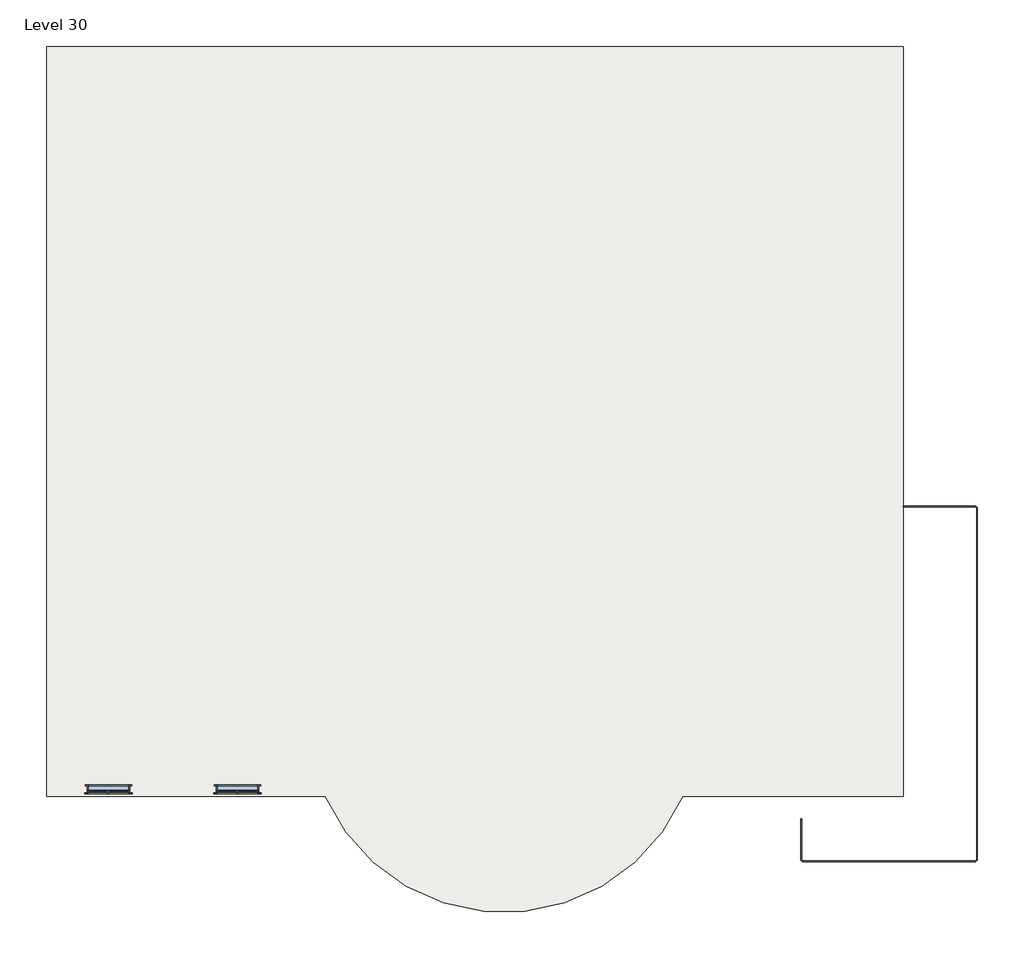
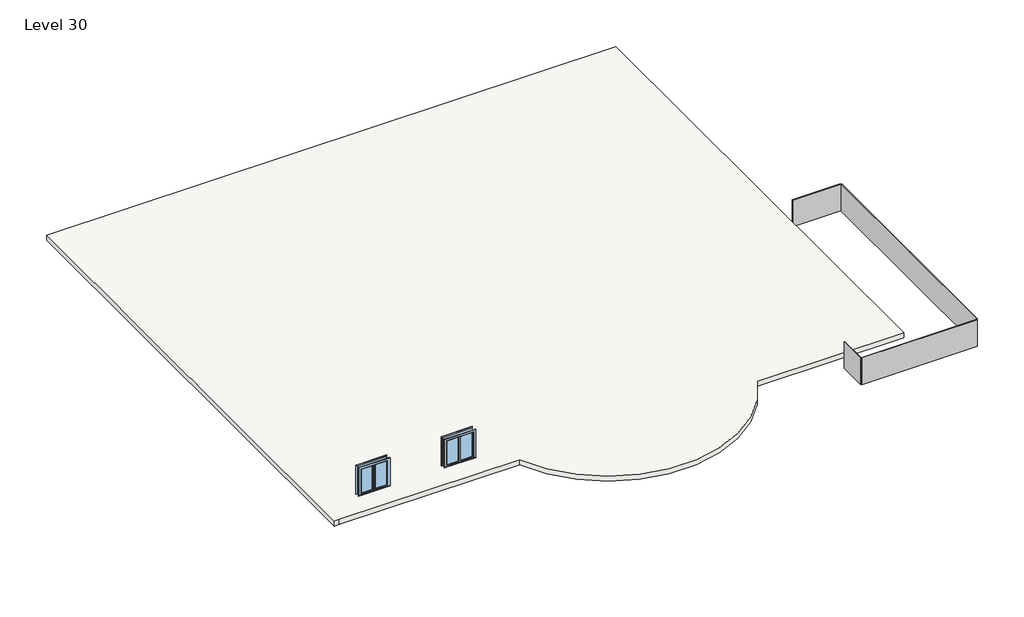
# One storey: 4 plates, 2 windows, 1 slab.
"""IFC4 building model written with IfcOpenShell, lengths in millimetres."""

from ifc_helpers import new_model, si_unit, point, frame, frame_2d, origin, place, context, project, spatial, polyline, circle_curve, trimmed, segment, composite_curve, outline, extrude, transform, mapped, element, save
from components import system_panel_glazed_4fcd3a06, system_panel_glazed_f6fb2dd6, system_panel_glazed_f39c722f, system_panel_glazed_542b97c0, window_0862ab64

model = new_model("IFC4")

# Units and contexts
model_context = context("Model", 3, world=origin())
ifc_project = project(units=[si_unit("LENGTHUNIT", "METRE", prefix="MILLI")], contexts=[model_context])

# Site, building, storey
site = spatial("IfcSite", under=ifc_project)
building = spatial("IfcBuilding", under=site)
storey = spatial("IfcBuildingStorey", under=building, Name="Level 30", Elevation=48920.4)

# Plates
placement = place(None, origin())
system_panel_glazed_shape = system_panel_glazed_4fcd3a06(model_context)
element("IfcPlate", 1, ObjectType="System Panel : Glazed", at=placement, inside=storey, context=model_context, shape_type="MappedRepresentation", body=[
    mapped(system_panel_glazed_shape, transform((9025.4464352, -5885.6278294, 48920.4), x_axis=(1.0, 0.0, 0.0), y_axis=(0.0, 1.0, 0.0), z_axis=(0.0, 0.0, 1.0))),
])
system_panel_glazed_2_shape = system_panel_glazed_f6fb2dd6(model_context)
element("IfcPlate", 2, ObjectType="System Panel : Glazed", at=placement, inside=storey, context=model_context, shape_type="MappedRepresentation", body=[
    mapped(system_panel_glazed_2_shape, transform((5082.0964352, -15423.3278294, 48920.4), x_axis=(0.0, 1.0, 0.0), y_axis=(-1.0, 0.0, 0.0), z_axis=(0.0, 0.0, 1.0))),
])
system_panel_glazed_3_shape = system_panel_glazed_f39c722f(model_context)
element("IfcPlate", 3, ObjectType="System Panel : Glazed", at=placement, inside=storey, context=model_context, shape_type="MappedRepresentation", body=[
    mapped(system_panel_glazed_3_shape, transform((10066.8464352, -10952.9278294, 48920.4), x_axis=(0.0, -1.0, 0.0), y_axis=(1.0, 0.0, 0.0), z_axis=(0.0, 0.0, 1.0))),
])
system_panel_glazed_4_shape = system_panel_glazed_542b97c0(model_context)
element("IfcPlate", 4, ObjectType="System Panel : Glazed", at=placement, inside=storey, context=model_context, shape_type="MappedRepresentation", body=[
    mapped(system_panel_glazed_4_shape, transform((7574.4714352, -16020.2278294, 48920.4), x_axis=(-1.0, 0.0, 0.0), y_axis=(0.0, -1.0, 0.0), z_axis=(0.0, 0.0, 1.0))),
])

# Slab
element("IfcSlab", 5, ObjectType="9\"", at=placement, inside=storey, context=model_context, shape_type="SweptSolid", body=[
    extrude(outline(composite_curve([segment(polyline([(-16607.9505427, 7350.6120962), (7979.2494573, 7350.6120962), (7979.2494573, -14188.5879038), (1652.8739931, -14188.5879038)]), True, "CONTINUOUS"), segment(trimmed(circle_curve(frame_2d((-3476.1505427, -11898.872104)), 5616.9111737), [point((1652.8739931, -14188.5879038))], [point((-8605.1750786, -14188.5879038))], False, "CARTESIAN"), True, "CONTINUOUS"), segment(polyline([(-8605.1750786, -14188.5879038), (-16404.7505427, -14188.5879038), (-16607.9505427, -14188.5879038), (-16607.9505427, 7350.6120962)]), True, "CONTINUOUS")], self_intersect=False)), frame((0.0, 0.0, 48915.3247039), z_axis=(0.0, 0.0, 1.0), x_axis=(1.0, 0.0, 0.0)), (0.0, 0.0, 1.0), 228.6),
])

# Windows
window_shape = window_0862ab64(model_context)
element("IfcWindow", 6, ObjectType="Casement Dbl with Trim : 48\" x 48\"", at=placement, inside=storey, context=model_context, shape_type="MappedRepresentation", body=[
    mapped(window_shape, transform((-14829.9505427, -13957.4308221, 48920.4), x_axis=(-1.0, 0.0, 0.0), y_axis=(0.0, -1.0, 0.0), z_axis=(0.0, 0.0, 1.0))),
])
element("IfcWindow", 7, ObjectType="Casement Dbl with Trim : 48\" x 48\"", at=placement, inside=storey, context=model_context, shape_type="MappedRepresentation", body=[
    mapped(window_shape, transform((-11129.6382271, -13957.4308221, 48920.4), x_axis=(-1.0, 0.0, 0.0), y_axis=(0.0, -1.0, 0.0), z_axis=(0.0, 0.0, 1.0))),
])

save(model, "model.ifc")

# Revit data of these elements
# Type "System Panel : Glazed"
#   Construction Type Id = "GSP4R"
#   Analytic Construction = "1/8 in Pilkington single glazing"
#   Visual Light Transmittance = 0.9
#   Solar Heat Gain Coefficient = 0.86
#   Heat Transfer Coefficient (U) = 1.18115 BTU/(h·ft²·°F)
# Type "9\""
#   Assembly Code = "B1010"
#   Function = 0
#   Layers, outside or top first: 0' - 9" no material (function 1)
# Type "Casement Dbl with Trim : 48\" x 48\""
#   Type Mark = "10"
#   Construction Type Id = "GSP4R"
#   Assembly Code = "B2020100"
#   Analytic Construction = "1/8 in Pilkington single glazing"
#   Visual Light Transmittance = 0.9
#   Solar Heat Gain Coefficient = 0.78
#   Heat Transfer Coefficient (U) = 0.6496 BTU/(h·ft²·°F)
#   Height = 4' - 0"
#   Default Sill Height = 3' - 0"
#   Trim Projection - Ext. = 0' - 0 1/2"
#   Trim Projection - Int. = 0' - 0 3/4"
#   Trim Width - Exterior = 0' - 3 1/2"
#   Trim Width - Interior = 0' - 3 1/2"
#   Width = 4' - 0"
#   Window Inset = 0' - 0 3/4"
#   Define Thermal Properties by = 1
#   Glass Pane Material = Glass
#   Sash Material = Sash
#   Trim Exterior Material = Trim
#   Trim Interior Material = Trim
#   Wall Closure = (empty or 0)
# Elements 1, 2, 3, 4 (IfcPlate, "System Panel : Glazed")
#   Phase Created = New Construction
#   Materials on its faces: "Glass"
# Element 5 (IfcSlab, "9\"")
#   built-in parameter 1001955 = 1.5708 (stored number, unit not read)
#   Height Offset From Level = 0' - 8.80019"
#   Phase Created = New Construction
#   Materials on its faces: "Default Floor"
# Element 6 (IfcWindow, "Casement Dbl with Trim : 48\" x 48\"")
#   Mark = "17"
#   Phase Created = New Construction
#   Materials on its faces: "Sash", "Trim", "Glass"
# Element 7 (IfcWindow, "Casement Dbl with Trim : 48\" x 48\"")
#   Mark = "18"
#   Phase Created = New Construction
#   Materials on its faces: "Sash", "Trim", "Glass"
# Materials
#   "Glass": class "Glass", colour RGB 0 128 192, transparency 0.75, Description = "Soda Lime Glass", Cost = 0
#   "Sash": class "Wood", colour RGB 224 178 126, transparency 0
#   "Trim": class "Wood", colour RGB 224 178 126, transparency 0
#   "Default Floor": colour RGB 128 128 128, transparency 0
